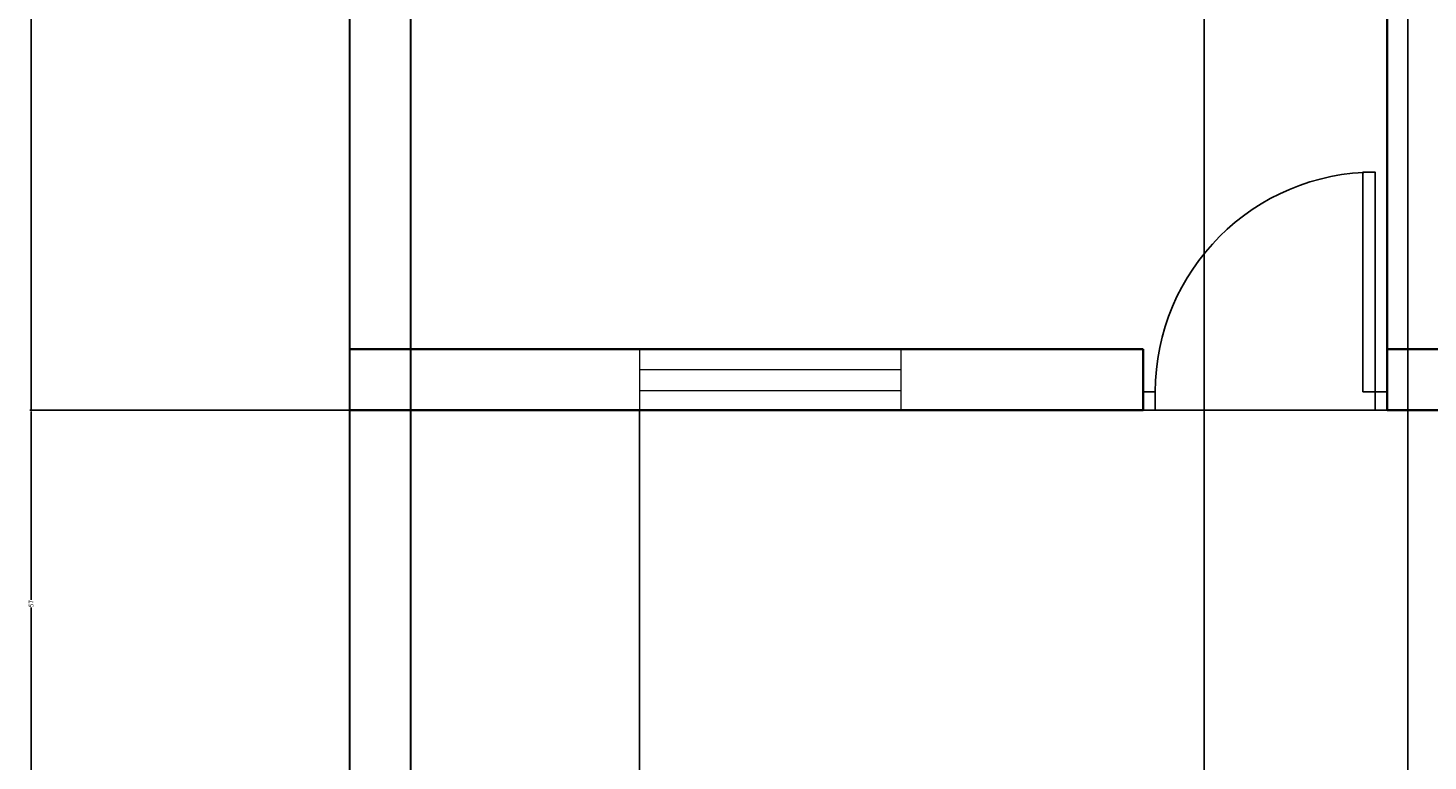
# Model space of a CAD drawing. Units: inches. Extents: x 867 to 1667, y -234 to 788.
# Tile 30 of 42: x 867 to 1074, y 572 to 680. Entities that reach past the tile are written whole.
import ezdxf

# ---------------------------------------------------------------- set-up
doc = ezdxf.new("R2010")
doc.units = ezdxf.units.IN
doc.header["$MEASUREMENT"] = 0
for name, color, linetype, lineweight in [('A-ANNO-DIMS', 2, 'Continuous', 18), ('A-Door', 150, 'Continuous', 25), ('A-Glaz', 92, 'Continuous', 18), ('A-Wall', 7, 'Continuous', 35), ('A-WALL-SITE', 8, 'Continuous', 30)]:
    doc.layers.add(name, color=color, linetype=linetype, lineweight=lineweight)
doc.layers.add('NET 01', color=8, linetype='Continuous')
doc.styles.get("Standard").update_dxf_attribs({"font": 'arial.ttf'})
doc.dimstyles.get("Standard").update_dxf_attribs({"dimtxt": 0.6875, "dimasz": 0.18, "dimexe": 0.18, "dimexo": 0.0625, "dimgap": 0.09, "dimtad": 0, "dimdec": 4, "dimzin": 0, "dimdsep": 46, "dimlunit": 4, "dimtxsty": 'Standard', "dimcen": 0.09, "dimadec": 0, "dimazin": 0, "dimtfac": 1, "dimtdec": 4, "dimtofl": 0, "dimtmove": 0, "dimatfit": 3, "dimfxl": 1, "dimtolj": 1, "dimtzin": 0, "dimarcsym": 0})

# ---------------------------------------------------------------- blocks, each defined once
blk = doc.blocks.new('A$C292B336C')
at = {"layer": 'A-Door'}
for points in [[(-0.05, 0), (-0.05, 0.9), (0, 0.9), (0, 0)], [(-0.95, 0), (-0.95, -0.075), (-0.9, -0.075), (-0.9, 0)], [(0, 0), (0, -0.075), (0.05, -0.075), (0.05, 0)]]:
    blk.add_lwpolyline(points, close=True, dxfattribs=at)
at = {"layer": 'NET 01'}
blk.add_arc((0, 0), 0.9, 90, 180, dxfattribs=at)
blk = doc.blocks.new('WIN-38_58IN')
for p, q in [((0, 9), (0, 0)), ((38.58, 0), (38.58, 9)), ((0, 6), (38.58, 6)), ((0, 2.92), (38.58, 2.92)), ((0, 0), (38.58, 0))]:
    blk.add_line(p, q)
blk = doc.blocks.new('*D19')
at = {"layer": 'A-ANNO-DIMS', "color": 0, "lineweight": -2, "transparency": 16777216}
for p, q in [((914.82, 740.62), (867.76, 740.62)), ((867.94, 740.44), (867.94, 682.93)), ((867.94, 623.8), (867.94, 681.3)), ((914.82, 623.62), (867.76, 623.62))]:
    blk.add_line(p, q, dxfattribs=at)
at = {"layer": 'A-ANNO-DIMS', "color": 0, "transparency": 16777216}
for points in [[(867.91, 740.44), (867.97, 740.44), (867.94, 740.62)], [(867.91, 623.8), (867.97, 623.8), (867.94, 623.62)]]:
    blk.add_solid(points, dxfattribs=at)
at = {"layer": 'Defpoints', "color": 0, "transparency": 16777216}
for p in [(867.94, 740.62), (914.89, 740.62), (914.89, 623.62)]:
    blk.add_point(p, dxfattribs=at)
at = {"layer": 'A-ANNO-DIMS', "color": 0, "transparency": 16777216, "insert": (867.94, 682.12), "char_height": 0.688, "attachment_point": 5, "rotation": 90}
blk.add_mtext('\\A1;117', dxfattribs=at)
blk = doc.blocks.new('*D24')
at = {"layer": 'A-ANNO-DIMS', "color": 0, "lineweight": -2, "transparency": 16777216}
for p, q in [((1067.82, 623.62), (867.76, 623.62)), ((867.94, 623.44), (867.94, 595.7)), ((867.94, 566.8), (867.94, 594.53)), ((1070.82, 566.62), (867.76, 566.62))]:
    blk.add_line(p, q, dxfattribs=at)
at = {"layer": 'A-ANNO-DIMS', "color": 0, "transparency": 16777216}
for points in [[(867.91, 623.44), (867.97, 623.44), (867.94, 623.62)], [(867.91, 566.8), (867.97, 566.8), (867.94, 566.62)]]:
    blk.add_solid(points, dxfattribs=at)
at = {"layer": 'Defpoints', "color": 0, "transparency": 16777216}
for p in [(1067.89, 623.62), (867.94, 566.62), (1070.89, 566.62)]:
    blk.add_point(p, dxfattribs=at)
at = {"layer": 'A-ANNO-DIMS', "color": 0, "transparency": 16777216, "insert": (867.94, 595.12), "char_height": 0.688, "attachment_point": 5, "rotation": 90}
blk.add_mtext('\\A1;57', dxfattribs=at)
blk = doc.blocks.new('*D28')
at = {"layer": 'A-ANNO-DIMS', "color": 0, "lineweight": -2, "transparency": 16777216}
for p, q in [((914.89, 623.55), (914.89, -233.54)), ((957.64, 623.55), (957.64, -233.54)), ((915.07, -233.36), (935, -233.36)), ((957.46, -233.36), (937.53, -233.36))]:
    blk.add_line(p, q, dxfattribs=at)
at = {"layer": 'A-ANNO-DIMS', "color": 0, "transparency": 16777216}
for points in [[(915.07, -233.33), (915.07, -233.39), (914.89, -233.36)], [(957.46, -233.33), (957.46, -233.39), (957.64, -233.36)]]:
    blk.add_solid(points, dxfattribs=at)
at = {"layer": 'Defpoints', "color": 0, "transparency": 16777216}
for p in [(914.89, 623.62), (957.64, 623.62), (914.89, -233.36)]:
    blk.add_point(p, dxfattribs=at)
at = {"layer": 'A-ANNO-DIMS', "color": 0, "transparency": 16777216, "insert": (936.26, -233.36), "char_height": 0.688, "attachment_point": 5}
blk.add_mtext('\\A1;42.75', dxfattribs=at)
blk = doc.blocks.new('*D31')
at = {"layer": 'A-ANNO-DIMS', "color": 0, "lineweight": -2, "transparency": 16777216}
for p, q in [((1070.89, 566.68), (1070.89, 787.75)), ((1071.07, 787.57), (1304.02, 787.57)), ((1538.71, 787.57), (1305.75, 787.57)), ((1538.89, 566.68), (1538.89, 787.75))]:
    blk.add_line(p, q, dxfattribs=at)
at = {"layer": 'A-ANNO-DIMS', "color": 0, "transparency": 16777216}
for points in [[(1071.07, 787.6), (1071.07, 787.54), (1070.89, 787.57)], [(1538.71, 787.6), (1538.71, 787.54), (1538.89, 787.57)]]:
    blk.add_solid(points, dxfattribs=at)
at = {"layer": 'Defpoints', "color": 0, "transparency": 16777216}
for p in [(1538.89, 787.57), (1070.89, 566.62), (1538.89, 566.62)]:
    blk.add_point(p, dxfattribs=at)
at = {"layer": 'A-ANNO-DIMS', "color": 0, "transparency": 16777216, "insert": (1304.89, 787.57), "char_height": 0.688, "attachment_point": 5}
blk.add_mtext('\\A1;468', dxfattribs=at)
blk = doc.blocks.new('*D35')
at = {"layer": 'A-ANNO-DIMS', "color": 0, "lineweight": -2, "transparency": 16777216}
for p, q in [((1040.89, 413.68), (1040.89, 787.75)), ((1041.07, 787.57), (1055.31, 787.57)), ((1070.71, 787.57), (1056.47, 787.57)), ((1070.89, 404.68), (1070.89, 787.75))]:
    blk.add_line(p, q, dxfattribs=at)
at = {"layer": 'A-ANNO-DIMS', "color": 0, "transparency": 16777216}
for points in [[(1041.07, 787.6), (1041.07, 787.54), (1040.89, 787.57)], [(1070.71, 787.6), (1070.71, 787.54), (1070.89, 787.57)]]:
    blk.add_solid(points, dxfattribs=at)
at = {"layer": 'Defpoints', "color": 0, "transparency": 16777216}
for p in [(1070.89, 787.57), (1040.89, 413.62), (1070.89, 404.62)]:
    blk.add_point(p, dxfattribs=at)
at = {"layer": 'A-ANNO-DIMS', "color": 0, "transparency": 16777216, "insert": (1055.89, 787.57), "char_height": 0.688, "attachment_point": 5}
blk.add_mtext('\\A1;30', dxfattribs=at)

msp = doc.modelspace()

# ---------------------------------------------------------------- linework, layer by layer
at = {"layer": 'A-Wall'}
for p, q in [((1067.8866, 740.617), (1067.8866, 623.617)), ((1031.8866, 632.617), (914.8866, 632.617)), ((1031.8866, 632.617), (1031.8866, 623.617)), ((1184.8866, 632.617), (1067.8866, 632.617)), ((1031.8866, 623.617), (914.8866, 623.617)), ((1186.5048, 623.617), (1067.8866, 623.617))]:
    msp.add_line(p, q, dxfattribs=at)
at = {"layer": 'A-WALL-SITE'}
for p, q in [((914.8866, 740.617), (914.8866, -186.4081)), ((923.8866, 740.617), (923.8866, -186.4081))]:
    msp.add_line(p, q, dxfattribs=at)

# ---------------------------------------------------------------- block references
at = {"layer": 'A-Door', "xscale": 36.01171521992244, "yscale": 36.01171521992244, "zscale": 36.01171521992244}
msp.add_blockref('A$C292B336C', (1066.086, 626.3179), dxfattribs=at)
at = {"layer": 'A-Glaz'}
msp.add_blockref('WIN-38_58IN', (957.638, 623.617), dxfattribs=at)

# ---------------------------------------------------------------- dimensions: what is measured, and where the dimension line sits
at = {"layer": 'A-ANNO-DIMS'}
for base, p1, p2, override, picture, middle in [((1070.8866, 787.567), (1040.8866, 413.617), (1070.8866, 404.617), {"dimdec": 0, "dimlfac": 1, "dimrnd": 0, "dimzin": 0, "dimdsep": 46, "dimlunit": 2}, '*D35', (1055.8866, 787.567)), ((1538.8866, 787.567), (1070.8866, 566.617), (1538.8866, 566.617), {"dimdec": 0, "dimlfac": 1, "dimrnd": 0, "dimzin": 0, "dimdsep": 46, "dimlunit": 2}, '*D31', (1304.8866, 787.567)), ((914.8866, -233.3581), (957.6375, 623.617), (914.8866, 623.617), {"dimdec": 2, "dimlfac": 1, "dimrnd": 0, "dimzin": 0, "dimdsep": 46, "dimlunit": 2}, '*D28', (936.2621, -233.3581))]:
    dim = msp.add_linear_dim(base=base, p1=p1, p2=p2, dimstyle='Standard', override=override, dxfattribs=at)
    dim.commit()
    dim.dimension.update_dxf_attribs({"geometry": picture, "text_midpoint": middle})
for base, p1, p2, picture, middle in [((867.9366, 740.617), (914.8866, 623.617), (914.8866, 740.617), '*D19', (867.9366, 682.117)), ((867.9366, 566.617), (1067.8866, 623.617), (1070.8866, 566.617), '*D24', (867.9366, 595.117))]:
    dim = msp.add_linear_dim(base=base, p1=p1, p2=p2, angle=90, dimstyle='Standard', override={"dimdec": 0, "dimlfac": 1, "dimrnd": 0, "dimzin": 0, "dimdsep": 46, "dimlunit": 2}, dxfattribs=at)
    dim.commit()
    dim.dimension.update_dxf_attribs({"geometry": picture, "text_midpoint": middle})

doc.saveas('drawing.dxf')
